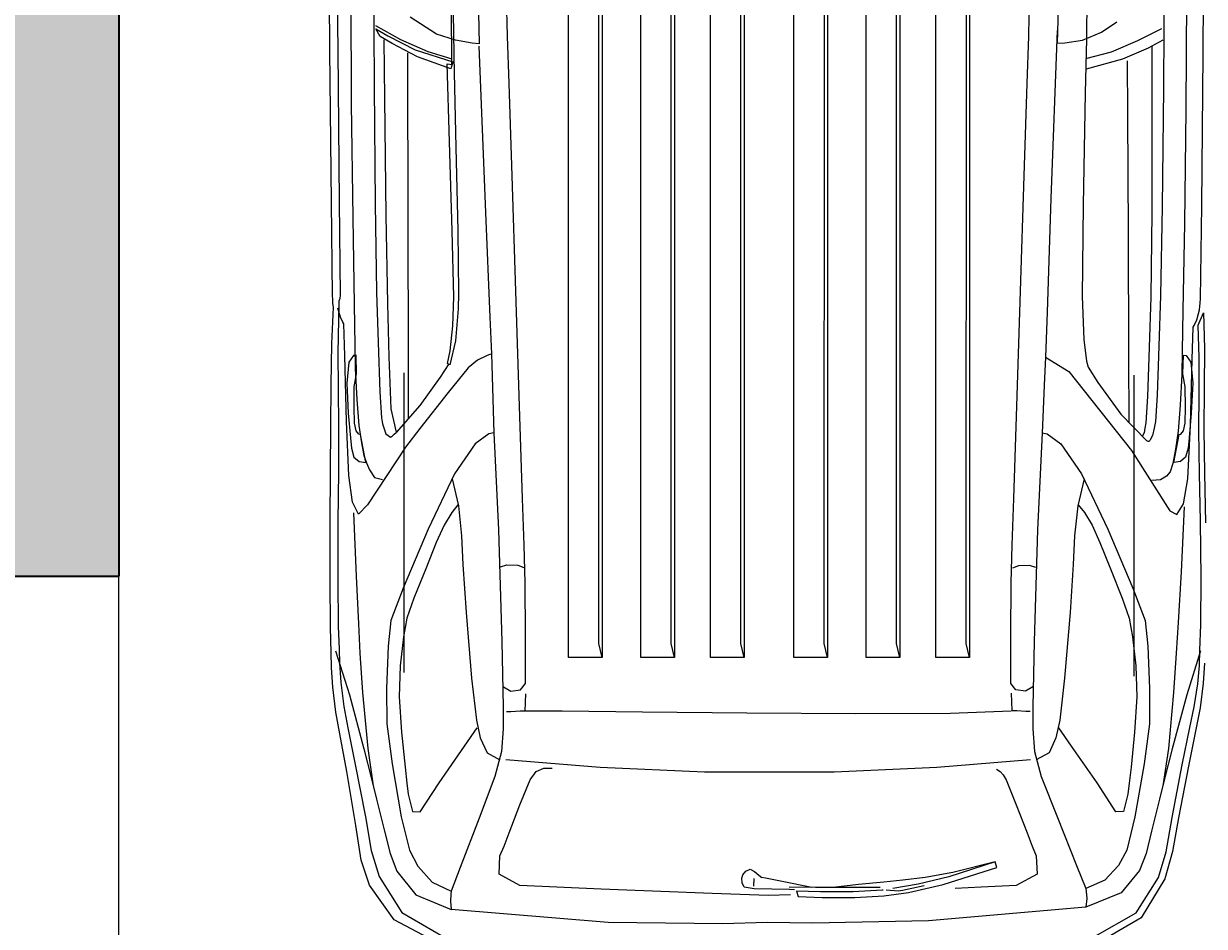
# Model space of a CAD drawing. Units: inches. Extents: x -16 to 587, y -783 to 64.
# Tile 3 of 14: x 111 to 195, y -697 to -633. Entities that reach past the tile are written whole.
import ezdxf

# ---------------------------------------------------------------- set-up
doc = ezdxf.new("R2010")
doc.units = ezdxf.units.IN
doc.header["$MEASUREMENT"] = 0
for name, color, linetype, lineweight in [('A-ANNO-DIMS', 2, 'Continuous', 18), ('A-SITE-VEHC', 8, 'Continuous', 13), ('A-WALL', 7, 'Continuous', 35), ('A-WALL-PATT', 23, 'Continuous', 13)]:
    doc.layers.add(name, color=color, linetype=linetype, lineweight=lineweight)
doc.styles.get("Standard").update_dxf_attribs({"font": 'arial.ttf'})
doc.dimstyles.get("Standard").update_dxf_attribs({"dimtxt": 0.18, "dimasz": 0.18, "dimexe": 0.18, "dimexo": 0.0625, "dimgap": 0.09, "dimtad": 0, "dimtih": 1, "dimtoh": 1, "dimdec": 0, "dimzin": 0, "dimdsep": 46, "dimlunit": 3, "dimtxsty": 'Standard', "dimcen": 0.09, "dimadec": 0, "dimazin": 0, "dimtfac": 1, "dimtdec": 0, "dimtofl": 0, "dimtmove": 0, "dimatfit": 3, "dimfxl": 1, "dimtolj": 1, "dimtzin": 0, "dimarcsym": 0})

# ---------------------------------------------------------------- blocks, each defined once
blk = doc.blocks.new('*D56')
at = {"layer": 'A-ANNO-DIMS', "color": 0, "lineweight": -2, "transparency": 16777216}
for p, q in [((118.083, -728.492), (118.083, 63.775)), ((228.083, -728.492), (228.083, 63.775)), ((118.263, 63.595), (172.753, 63.595)), ((227.903, 63.595), (173.412, 63.595))]:
    blk.add_line(p, q, dxfattribs=at)
at = {"layer": 'A-ANNO-DIMS', "color": 0, "transparency": 16777216}
for points in [[(118.263, 63.625), (118.263, 63.565), (118.083, 63.595)], [(227.903, 63.625), (227.903, 63.565), (228.083, 63.595)]]:
    blk.add_solid(points, dxfattribs=at)
at = {"layer": 'Defpoints', "color": 0, "transparency": 16777216}
for p in [(228.083, 63.595), (118.083, -728.555), (228.083, -728.555)]:
    blk.add_point(p, dxfattribs=at)
at = {"layer": 'A-ANNO-DIMS', "color": 0, "transparency": 16777216, "insert": (173.083, 63.595), "char_height": 0.18, "attachment_point": 5}
blk.add_mtext('\\A1;9\'-2"', dxfattribs=at)

msp = doc.modelspace()

# ---------------------------------------------------------------- hatches: boundary and pattern name
at = {"layer": 'A-WALL-PATT'}
h = msp.add_hatch(color=256, dxfattribs=at)
h.dxf.hatch_style = 1
h.paths.add_polyline_path([(137.083, -543.555), (137.083, -534.555), (118.083, -534.555), (118.083, -528.555), (109.083, -528.555), (109.083, -534.555), (109.083, -672.555), (118.083, -672.555), (118.083, -543.555)], flags=17)
h.paths.add_polyline_path([(27.083, -663.555), (27.083, -400.555), (73.083, -400.555), (73.083, -391.555), (27.083, -391.555), (27.083, 10.445), (48.751, 10.445), (171.083, 10.445), (171.083, -17.555), (180.083, -17.555), (180.083, 10.445), (228.083, 10.445), (228.083, -262.555), (206.414, -262.555), (118.083, -262.555), (118.083, -271.555), (228.083, -271.555), (228.083, -391.555), (154.083, -391.555), (154.083, -400.555), (228.083, -400.555), (228.083, -534.555), (209.083, -534.555), (209.083, -543.555), (237.083, -543.555), (237.083, 19.445), (18.083, 19.445), (18.083, -672.555), (73.083, -672.555), (73.083, -663.555)])
h.paths.add_polyline_path([(109.083, -486.555), (87.083, -486.555), (87.083, -495.555), (118.083, -495.555), (118.083, -400.555), (118.083, -391.555), (109.083, -391.555), (109.083, -400.555)], flags=17)

# ---------------------------------------------------------------- linework, layer by layer
at = {"layer": 'A-SITE-VEHC'}
for p, q in [((149.989, -678.315), (149.989, -615.867)), ((152.131, -677.322), (152.153, -616.064)), ((152.368, -615.867), (152.368, -678.315)), ((152.369, -615.867), (152.369, -678.315)), ((155.117, -678.315), (155.117, -615.867)), ((157.258, -677.322), (157.281, -616.064)), ((157.495, -615.867), (157.495, -678.315)), ((157.497, -615.867), (157.497, -678.315)), ((160.061, -678.315), (160.061, -615.867)), ((162.203, -677.322), (162.226, -616.064)), ((162.44, -615.867), (162.44, -678.315)), ((162.442, -615.867), (162.442, -678.315)), ((165.977, -678.315), (165.977, -615.867)), ((168.119, -677.322), (168.142, -616.064)), ((168.355, -615.867), (168.355, -678.315)), ((168.358, -615.867), (168.358, -678.315)), ((171.105, -678.315), (171.105, -615.867)), ((173.247, -677.322), (173.269, -616.064)), ((173.483, -615.867), (173.483, -678.315)), ((173.485, -615.867), (173.485, -678.315)), ((176.049, -678.315), (176.049, -615.867)), ((178.193, -677.322), (178.216, -616.064)), ((178.43, -615.867), (178.43, -678.315)), ((136.149, -628.168), (136.172, -633.662)), ((143.513, -627.927), (143.651, -634.79)), ((184.831, -628.18), (184.658, -634.742)), ((186.781, -628.18), (186.726, -634.447)), ((192.201, -628.493), (192.219, -633.733)), ((133.062, -635.266), (133.014, -629.627)), ((133.563, -629.627), (133.612, -635.26)), ((134.53, -630.409), (134.576, -639.048)), ((195.007, -635.526), (195.055, -629.894)), ((145.651, -634.256), (145.592, -631.197)), ((182.649, -634.256), (182.694, -631.197)), ((193.822, -630.822), (193.776, -639.461)), ((141.7, -636.249), (141.678, -632.257)), ((141.81, -632.032), (141.839, -634.647)), ((140.613, -634.097), (138.765, -632.909)), ((187.79, -633.974), (188.879, -633.219)), ((136.172, -633.662), (136.195, -637.823)), ((136.3, -633.494), (138.077, -634.49)), ((136.629, -634.28), (136.309, -633.731)), ((136.309, -633.731), (137.18, -634.234)), ((184.654, -633.854), (184.211, -645.765)), ((186.45, -634.523), (187.79, -633.974)), ((192.055, -633.715), (190.357, -634.583)), ((192.219, -633.733), (192.184, -637.941)), ((137.472, -634.762), (136.629, -634.28)), ((136.881, -634.509), (136.926, -638.662)), ((137.18, -634.234), (139.112, -635.22)), ((139.269, -635.713), (137.472, -634.762)), ((138.077, -634.49), (139.998, -635.336)), ((141.97, -634.541), (140.613, -634.097)), ((141.839, -634.647), (141.844, -634.913)), ((141.844, -634.913), (141.858, -635.662)), ((143.148, -634.743), (141.97, -634.541)), ((143.651, -634.79), (143.148, -634.743)), ((145.773, -637.594), (145.651, -634.256)), ((182.528, -637.594), (182.649, -634.256)), ((184.658, -634.742), (185.206, -634.718)), ((185.206, -634.718), (186.45, -634.523)), ((186.726, -634.447), (186.648, -638.301)), ((190.357, -634.583), (188.471, -635.385)), ((191.135, -635.064), (192.159, -634.504)), ((133.163, -646.019), (133.062, -635.266)), ((133.612, -635.26), (133.712, -646.003)), ((138.575, -635.425), (138.591, -647.803)), ((139.112, -635.22), (141.791, -636.078)), ((141.632, -636.568), (139.269, -635.713)), ((139.998, -635.336), (141.711, -635.86)), ((141.858, -635.662), (141.879, -636.817)), ((143.633, -634.947), (144.098, -646.751)), ((188.471, -635.385), (186.667, -635.865)), ((189.312, -635.852), (191.135, -635.064)), ((191.363, -634.99), (191.372, -638.895)), ((194.907, -646.267), (195.007, -635.526)), ((141.541, -641.747), (141.368, -636.203)), ((141.368, -636.203), (141.7, -636.249)), ((141.791, -636.078), (141.632, -636.568)), ((186.726, -636.575), (189.312, -635.852)), ((189.624, -635.997), (189.641, -639.778)), ((141.879, -636.817), (141.997, -642.132)), ((136.195, -637.823), (136.26, -646.146)), ((145.986, -644.154), (145.773, -637.594)), ((182.315, -644.154), (182.528, -637.594)), ((192.184, -637.941), (192.096, -646.352)), ((134.576, -639.048), (134.677, -647.128)), ((136.926, -638.662), (137.032, -646.97)), ((186.648, -638.301), (186.504, -646.213)), ((191.372, -638.895), (191.366, -646.746)), ((189.641, -639.778), (189.68, -648.216)), ((193.776, -639.461), (193.674, -647.541)), ((141.737, -648.057), (141.541, -641.747)), ((141.997, -642.132), (142.129, -648.027)), ((146.246, -652.323), (145.986, -644.154)), ((182.055, -652.323), (182.315, -644.154)), ((184.211, -645.765), (183.932, -653.817)), ((133.251, -652.643), (133.163, -646.019)), ((133.712, -646.003), (133.8, -652.621)), ((136.26, -646.146), (136.362, -652.395)), ((186.504, -646.213), (186.427, -652.707)), ((192.096, -646.352), (191.982, -652.648)), ((194.819, -652.885), (194.907, -646.267)), ((134.677, -647.128), (134.779, -653.29)), ((137.032, -646.97), (137.156, -653.211)), ((144.098, -646.751), (144.407, -654.185)), ((191.366, -646.746), (191.295, -652.74)), ((138.591, -647.803), (138.603, -656.65)), ((141.849, -652.731), (141.737, -648.057)), ((142.129, -648.027), (142.192, -652.466)), ((189.68, -648.216), (189.719, -656.953)), ((193.674, -647.541), (193.573, -653.703)), ((136.362, -652.395), (136.48, -655.983)), ((142.192, -652.466), (142.151, -653.59)), ((146.506, -660.487), (146.246, -652.323)), ((181.795, -660.487), (182.055, -652.323)), ((133.259, -652.922), (133.251, -652.643)), ((133.272, -653.202), (133.259, -652.922)), ((133.306, -653.479), (133.272, -653.202)), ((133.699, -653.28), (133.676, -654.356)), ((133.705, -653.053), (133.699, -653.28)), ((133.767, -652.85), (133.705, -653.053)), ((133.8, -652.621), (133.767, -652.85)), ((134.779, -653.29), (134.825, -656.178)), ((137.156, -653.211), (137.246, -656.981)), ((141.779, -654.797), (141.849, -652.731)), ((186.427, -652.707), (186.534, -655.77)), ((191.295, -652.74), (191.177, -656.327)), ((191.982, -652.648), (191.864, -656.236)), ((194.776, -653.424), (194.802, -653.167)), ((194.802, -653.167), (194.819, -652.885)), ((133.208, -656.064), (133.306, -653.479)), ((133.807, -654.176), (133.626, -653.534)), ((133.98, -654.532), (133.807, -654.176)), ((142.151, -653.59), (141.974, -655.847)), ((183.932, -653.817), (183.827, -657.007)), ((193.573, -653.703), (193.527, -656.591)), ((194.557, -654.376), (194.742, -653.659)), ((194.66, -654.745), (195.036, -653.862)), ((194.742, -653.659), (194.776, -653.424)), ((195.036, -653.862), (195.093, -656.392)), ((133.676, -654.356), (133.624, -656.711)), ((134.057, -654.641), (133.98, -654.532)), ((134.109, -656.918), (134.057, -654.641)), ((141.592, -656.558), (141.779, -654.797)), ((144.407, -654.185), (144.518, -656.769)), ((194.235, -657.171), (194.287, -654.894)), ((194.287, -654.894), (194.371, -654.773)), ((194.371, -654.773), (194.557, -654.376)), ((194.724, -657.068), (194.66, -654.745)), ((141.974, -655.847), (141.574, -657.56)), ((186.534, -655.77), (186.733, -657.308)), ((133.148, -658.988), (133.208, -656.064)), ((134.825, -656.178), (134.862, -657.82)), ((136.48, -655.983), (136.598, -659.466)), ((138.603, -656.65), (138.608, -661.379)), ((141.391, -657.469), (141.592, -656.558)), ((191.177, -656.327), (191.059, -659.81)), ((191.864, -656.236), (191.746, -659.719)), ((193.527, -656.591), (193.489, -658.233)), ((195.093, -656.392), (195.072, -659.213)), ((133.624, -656.711), (133.652, -659.212)), ((134.241, -661.585), (134.109, -656.918)), ((134.405, -657.373), (134.258, -658.856)), ((134.739, -656.903), (134.405, -657.373)), ((134.924, -656.874), (134.739, -656.903)), ((134.957, -658.2), (134.924, -656.874)), ((137.246, -656.981), (137.389, -660.687)), ((141.504, -657.478), (140.893, -658.423)), ((141.574, -657.56), (141.391, -657.469)), ((143.54, -657.231), (142.863, -657.774)), ((144.169, -656.915), (143.54, -657.231)), ((144.446, -656.813), (144.169, -656.915)), ((144.518, -656.769), (144.7, -662.379)), ((183.827, -657.007), (183.737, -659.007)), ((183.827, -657.007), (185.481, -658.027)), ((186.733, -657.308), (186.84, -657.731)), ((189.719, -656.953), (189.736, -661.632)), ((193.573, -658.2), (193.607, -656.874)), ((193.607, -656.874), (193.792, -656.903)), ((193.792, -656.903), (194.125, -657.373)), ((194.103, -661.837), (194.235, -657.171)), ((194.125, -657.373), (194.273, -658.856)), ((194.72, -659.512), (194.724, -657.068)), ((134.789, -659.128), (134.957, -658.2)), ((134.862, -657.82), (134.965, -660.013)), ((138.299, -658.133), (138.299, -679.377)), ((142.863, -657.774), (141.451, -659.518)), ((185.481, -658.027), (189.913, -663.641)), ((186.84, -657.731), (187.545, -658.817)), ((190.084, -658.285), (190.084, -679.645)), ((193.489, -658.233), (193.387, -660.426)), ((193.741, -659.128), (193.573, -658.2)), ((133.129, -661.962), (133.148, -658.988)), ((134.258, -658.856), (134.367, -660.989)), ((134.783, -660.566), (134.789, -659.128)), ((140.893, -658.423), (139.45, -660.453)), ((183.737, -659.007), (183.634, -661.29)), ((187.545, -658.817), (189.169, -661.058)), ((193.748, -660.566), (193.741, -659.128)), ((194.273, -658.856), (194.164, -660.989)), ((133.652, -659.212), (133.678, -661.962)), ((134.965, -660.013), (135.121, -661.852)), ((136.598, -659.466), (136.716, -661.32)), ((141.451, -659.518), (139.448, -662.077)), ((191.059, -659.81), (190.941, -661.664)), ((191.746, -659.719), (191.628, -661.573)), ((194.706, -662.231), (194.72, -659.512)), ((195.072, -659.213), (195.049, -662.139)), ((134.809, -661.704), (134.783, -660.566)), ((137.389, -660.687), (137.751, -662.323)), ((139.45, -660.453), (137.754, -662.366)), ((146.72, -667.033), (146.506, -660.487)), ((181.581, -667.033), (181.795, -660.487)), ((193.387, -660.426), (193.231, -662.265)), ((193.722, -661.704), (193.748, -660.566)), ((134.412, -665.398), (134.241, -661.585)), ((134.367, -660.989), (134.512, -662.738)), ((134.916, -662.248), (134.809, -661.704)), ((136.716, -661.32), (136.794, -661.737)), ((183.634, -661.29), (183.584, -662.379)), ((189.169, -661.058), (190.978, -662.932)), ((190.941, -661.664), (190.88, -662.049)), ((191.628, -661.573), (191.533, -662.053)), ((193.615, -662.248), (193.722, -661.704)), ((194.164, -660.989), (194.019, -662.738)), ((133.113, -665.101), (133.129, -661.962)), ((133.678, -661.962), (133.663, -665.101)), ((135.115, -662.466), (134.916, -662.248)), ((135.221, -662.505), (135.115, -662.466)), ((135.121, -661.852), (135.298, -663.08)), ((135.61, -664.497), (135.221, -662.505)), ((136.794, -661.737), (137.017, -662.456)), ((137.017, -662.456), (137.367, -662.679)), ((137.493, -662.585), (137.623, -662.48)), ((137.623, -662.48), (137.754, -662.366)), ((139.448, -662.077), (138.431, -663.388)), ((144.346, -662.447), (143.37, -663.163)), ((144.7, -662.379), (144.346, -662.447)), ((144.7, -662.379), (145.028, -669.269)), ((183.584, -662.379), (183.256, -669.269)), ((183.584, -662.379), (183.939, -662.447)), ((183.939, -662.447), (184.915, -663.163)), ((190.821, -662.384), (190.677, -662.643)), ((190.88, -662.049), (190.821, -662.384)), ((191.533, -662.053), (191.41, -662.566)), ((192.92, -664.497), (193.309, -662.505)), ((193.231, -662.265), (193.046, -663.548)), ((193.309, -662.505), (193.416, -662.466)), ((193.416, -662.466), (193.615, -662.248)), ((193.932, -665.651), (194.103, -661.837)), ((194.747, -665.254), (194.706, -662.231)), ((195.049, -662.139), (195.092, -665.231)), ((134.512, -662.738), (134.584, -663.462)), ((135.298, -663.08), (135.475, -663.992)), ((138.431, -663.388), (135.737, -667.496)), ((137.367, -662.679), (137.493, -662.585)), ((143.37, -663.163), (141.906, -665.292)), ((184.915, -663.163), (186.379, -665.292)), ((190.978, -662.932), (191.072, -662.976)), ((191.072, -662.976), (191.157, -662.97)), ((191.157, -662.97), (191.231, -662.921)), ((191.41, -662.566), (191.231, -662.921)), ((194.019, -662.738), (193.947, -663.462)), ((134.584, -663.462), (134.769, -664.1)), ((134.769, -664.1), (135.126, -664.407)), ((135.475, -663.992), (135.653, -664.511)), ((189.913, -663.641), (192.645, -667.908)), ((193.046, -663.548), (192.854, -664.564)), ((193.761, -664.1), (193.404, -664.407)), ((193.947, -663.462), (193.761, -664.1)), ((135.126, -664.407), (135.61, -664.497)), ((135.653, -664.511), (135.874, -664.998)), ((135.874, -664.998), (136.229, -665.55)), ((192.854, -664.564), (192.668, -665.138)), ((193.404, -664.407), (192.92, -664.497)), ((133.085, -668.714), (133.113, -665.101)), ((133.663, -665.101), (133.634, -668.714)), ((134.666, -667.307), (134.412, -665.398)), ((136.229, -665.55), (136.79, -665.687)), ((141.906, -665.292), (140.034, -669.218)), ((141.727, -665.649), (142.179, -667.552)), ((186.557, -665.649), (186.106, -667.552)), ((186.379, -665.292), (188.251, -669.218)), ((191.988, -665.712), (191.363, -665.756)), ((192.414, -665.455), (191.988, -665.712)), ((192.668, -665.138), (192.414, -665.455)), ((193.617, -667.426), (193.932, -665.651)), ((194.824, -668.655), (194.747, -665.254)), ((195.092, -665.231), (195.172, -668.76)), ((135.097, -668.146), (134.666, -667.307)), ((135.737, -667.496), (135.097, -668.146)), ((142.143, -667.492), (141.703, -668.027)), ((142.179, -667.552), (142.406, -669.692)), ((146.841, -670.346), (146.72, -667.033)), ((181.46, -670.346), (181.581, -667.033)), ((186.106, -667.552), (185.879, -669.692)), ((186.141, -667.492), (186.581, -668.027)), ((193.133, -668.165), (193.617, -667.426)), ((134.729, -668.045), (134.914, -672.546)), ((141.703, -668.027), (141.157, -668.919)), ((186.581, -668.027), (187.128, -668.919)), ((192.645, -667.908), (193.133, -668.165)), ((193.653, -667.633), (193.443, -672.241)), ((133.069, -672.843), (133.085, -668.714)), ((133.634, -668.714), (133.619, -672.843)), ((140.034, -669.218), (138.268, -673.396)), ((141.157, -668.919), (140.598, -670.168)), ((187.128, -668.919), (187.687, -670.168)), ((188.251, -669.218), (190.017, -673.396)), ((194.866, -672.669), (194.824, -668.655)), ((142.406, -669.692), (142.5, -671.714)), ((145.028, -669.269), (145.264, -677.19)), ((183.256, -669.269), (183.021, -677.19)), ((185.879, -669.692), (185.784, -671.714)), ((140.598, -670.168), (139.86, -672.017)), ((146.907, -673.014), (146.841, -670.346)), ((181.394, -673.014), (181.46, -670.346)), ((187.687, -670.168), (188.425, -672.017)), ((142.5, -671.714), (142.72, -675.136)), ((145.168, -671.891), (145.601, -671.753)), ((145.601, -671.753), (146.402, -671.759)), ((146.402, -671.759), (146.828, -671.925)), ((185.784, -671.714), (185.564, -675.136)), ((134.914, -672.546), (135.082, -675.933)), ((139.86, -672.017), (139.017, -674.105)), ((181.898, -671.805), (181.473, -671.971)), ((182.7, -671.798), (181.898, -671.805)), ((183.133, -671.937), (182.7, -671.798)), ((188.425, -672.017), (189.268, -674.105)), ((193.443, -672.241), (193.228, -675.826)), ((133.096, -676.179), (133.069, -672.843)), ((133.619, -672.843), (133.65, -676.1)), ((138.268, -673.396), (137.387, -675.697)), ((146.938, -676.737), (146.907, -673.014)), ((181.363, -676.737), (181.394, -673.014)), ((190.017, -673.396), (190.897, -675.697)), ((194.836, -676.009), (194.866, -672.669)), ((139.017, -674.105), (138.517, -675.519)), ((189.268, -674.105), (189.768, -675.519)), ((135.082, -675.933), (135.187, -678.016)), ((137.387, -675.697), (137.204, -677.514)), ((138.517, -675.519), (138.286, -676.849)), ((142.72, -675.136), (143.112, -679.786)), ((185.564, -675.136), (185.172, -679.786)), ((189.768, -675.519), (189.999, -676.849)), ((190.897, -675.697), (191.08, -677.514)), ((193.228, -675.826), (193.098, -678.016)), ((133.146, -677.957), (133.096, -676.179)), ((133.65, -676.1), (133.707, -677.732)), ((146.939, -680.172), (146.938, -676.737)), ((181.362, -680.172), (181.363, -676.737)), ((194.781, -677.793), (194.836, -676.009)), ((137.204, -677.514), (137.074, -680.519)), ((138.286, -676.849), (138.054, -678.905)), ((145.264, -677.19), (145.354, -681.821)), ((152.368, -678.315), (152.131, -677.322)), ((157.495, -678.315), (157.258, -677.322)), ((162.44, -678.315), (162.203, -677.322)), ((168.355, -678.315), (168.119, -677.322)), ((173.483, -678.315), (173.247, -677.322)), ((178.43, -678.315), (178.193, -677.322)), ((183.021, -677.19), (182.93, -681.821)), ((189.999, -676.849), (190.23, -678.905)), ((191.08, -677.514), (191.21, -680.519)), ((133.173, -679.033), (133.146, -677.957)), ((133.463, -677.837), (134.443, -680.962)), ((133.707, -677.732), (133.738, -678.729)), ((135.187, -678.016), (135.381, -680.808)), ((152.369, -678.315), (149.989, -678.315)), ((157.497, -678.315), (155.117, -678.315)), ((162.442, -678.315), (160.061, -678.315)), ((168.358, -678.315), (165.977, -678.315)), ((173.485, -678.315), (171.105, -678.315)), ((178.43, -678.315), (176.049, -678.315)), ((193.098, -678.016), (192.904, -680.808)), ((194.822, -677.837), (193.842, -680.962)), ((194.751, -678.873), (194.781, -677.793)), ((133.262, -680.431), (133.173, -679.033)), ((133.738, -678.729), (133.825, -680.08)), ((138.054, -678.905), (137.982, -681.107)), ((190.23, -678.905), (190.303, -681.107)), ((194.638, -680.183), (194.751, -678.873)), ((195.096, -678.729), (195.007, -680.127)), ((133.825, -680.08), (134.042, -681.789)), ((143.112, -679.786), (143.452, -682.772)), ((185.172, -679.786), (184.833, -682.772)), ((195.007, -680.127), (194.784, -681.879)), ((133.485, -682.183), (133.262, -680.431)), ((134.443, -680.962), (135.476, -684.8)), ((135.381, -680.808), (135.746, -684.776)), ((137.074, -680.519), (137.09, -683.01)), ((145.378, -680.4), (145.888, -680.709)), ((145.888, -680.709), (146.587, -680.61)), ((146.587, -680.61), (146.939, -680.172)), ((146.939, -680.899), (146.9, -682.118)), ((181.714, -680.61), (181.362, -680.172)), ((181.397, -680.848), (181.436, -682.068)), ((182.413, -680.709), (181.714, -680.61)), ((182.923, -680.4), (182.413, -680.709)), ((191.21, -680.519), (191.195, -683.01)), ((192.904, -680.808), (192.538, -684.776)), ((193.842, -680.962), (192.809, -684.8)), ((194.373, -681.818), (194.638, -680.183)), ((134.042, -681.789), (134.325, -683.303)), ((137.982, -681.107), (138.147, -683.62)), ((145.354, -681.821), (145.359, -683.365)), ((182.93, -681.821), (182.926, -683.365)), ((190.303, -681.107), (190.138, -683.62)), ((194.065, -683.291), (194.373, -681.818)), ((133.775, -683.735), (133.485, -682.183)), ((145.905, -682.162), (145.592, -682.178)), ((146.548, -682.134), (145.905, -682.162)), ((146.9, -682.118), (146.548, -682.134)), ((149.539, -682.131), (146.9, -682.118)), ((155.239, -682.197), (149.539, -682.131)), ((162.637, -682.274), (155.239, -682.197)), ((170.37, -682.316), (162.637, -682.274)), ((177.073, -682.279), (170.37, -682.316)), ((181.384, -682.118), (177.073, -682.279)), ((181.436, -682.068), (181.789, -682.083)), ((181.789, -682.083), (182.432, -682.112)), ((182.432, -682.112), (182.744, -682.127)), ((194.784, -681.879), (194.494, -683.43)), ((134.325, -683.303), (134.864, -685.906)), ((137.09, -683.01), (137.466, -685.866)), ((142.608, -684.598), (143.511, -683.307)), ((143.452, -682.772), (143.725, -684.012)), ((145.359, -683.365), (145.231, -684.974)), ((182.926, -683.365), (183.054, -684.974)), ((184.833, -682.772), (184.56, -684.012)), ((185.676, -684.598), (184.774, -683.307)), ((191.195, -683.01), (190.818, -685.866)), ((193.525, -685.921), (194.065, -683.291)), ((194.494, -683.43), (193.959, -686.016)), ((134.273, -686.4), (133.775, -683.735)), ((138.147, -683.62), (138.391, -686.106)), ((143.725, -684.012), (144.209, -685.08)), ((184.56, -684.012), (184.076, -685.08)), ((190.138, -683.62), (189.893, -686.106)), ((135.476, -684.8), (136.02, -686.934)), ((135.746, -684.776), (136.138, -687.41)), ((140.807, -687.209), (142.608, -684.598)), ((144.209, -685.08), (145.116, -685.567)), ((145.231, -684.974), (144.76, -686.756)), ((183.054, -684.974), (183.525, -686.756)), ((184.076, -685.08), (183.168, -685.567)), ((187.478, -687.209), (185.676, -684.598)), ((192.538, -684.776), (192.146, -687.41)), ((192.809, -684.8), (192.265, -686.934)), ((134.864, -685.906), (135.575, -689.609)), ((137.466, -685.866), (138.12, -689.608)), ((152.225, -686.128), (145.532, -685.567)), ((182.752, -685.567), (176.122, -686.128)), ((190.818, -685.866), (190.164, -689.608)), ((192.813, -689.674), (193.525, -685.921)), ((134.909, -690.228), (134.273, -686.4)), ((138.391, -686.106), (138.517, -687.231)), ((144.76, -686.756), (143.641, -689.711)), ((147.257, -686.994), (147.685, -686.399)), ((147.685, -686.399), (148.228, -686.165)), ((148.228, -686.165), (148.83, -686.159)), ((159.63, -686.452), (152.225, -686.128)), ((164.261, -686.458), (159.63, -686.452)), ((168.831, -686.452), (164.261, -686.458)), ((176.122, -686.128), (168.831, -686.452)), ((180.337, -686.245), (180.599, -686.398)), ((180.599, -686.398), (180.831, -686.642)), ((180.831, -686.642), (181.028, -686.994)), ((183.525, -686.756), (184.663, -689.664)), ((189.893, -686.106), (189.768, -687.231)), ((193.959, -686.016), (193.252, -689.694)), ((136.02, -686.934), (136.372, -688.359)), ((138.517, -687.231), (138.618, -688.007)), ((139.468, -689.253), (140.807, -687.209)), ((146.541, -688.766), (147.257, -686.994)), ((181.028, -686.994), (181.744, -688.766)), ((188.817, -689.253), (187.478, -687.209)), ((189.768, -687.231), (189.667, -688.007)), ((192.265, -686.934), (191.913, -688.359)), ((136.372, -688.359), (136.936, -690.642)), ((138.618, -688.007), (138.931, -689.231)), ((189.667, -688.007), (189.354, -689.231)), ((191.913, -688.359), (191.349, -690.642)), ((138.931, -689.231), (139.468, -689.253)), ((145.773, -690.751), (146.541, -688.766)), ((181.744, -688.766), (182.512, -690.751)), ((189.354, -689.231), (188.817, -689.253)), ((135.575, -689.609), (135.995, -692.013)), ((138.12, -689.608), (138.695, -691.988)), ((143.641, -689.711), (142.311, -693.207)), ((184.663, -689.664), (186.031, -693.071)), ((190.164, -689.608), (189.59, -691.988)), ((192.393, -692.104), (192.813, -689.674)), ((193.252, -689.694), (192.835, -692.082)), ((135.289, -692.696), (134.909, -690.228)), ((136.936, -690.642), (137.328, -692.226)), ((145.414, -691.691), (145.773, -690.751)), ((182.512, -690.751), (182.871, -691.691)), ((191.349, -690.642), (190.957, -692.226)), ((145.112, -692.376), (145.414, -691.691)), ((182.871, -691.691), (183.173, -692.376)), ((135.879, -694.476), (135.289, -692.696)), ((135.995, -692.013), (136.555, -693.85)), ((137.328, -692.226), (137.815, -693.481)), ((138.695, -691.988), (139.307, -693.111)), ((145.061, -693.681), (145.112, -692.376)), ((183.173, -692.376), (183.223, -693.681)), ((189.59, -691.988), (188.997, -693.064)), ((190.957, -692.226), (190.49, -693.434)), ((191.845, -693.911), (192.393, -692.104)), ((192.835, -692.082), (192.287, -694.021)), ((137.815, -693.481), (139.148, -695.144)), ((139.307, -693.111), (140.303, -694.246)), ((142.311, -693.207), (141.668, -694.894)), ((162.353, -693.728), (162.566, -693.46)), ((162.566, -693.46), (162.864, -693.341)), ((162.864, -693.341), (163.191, -693.491)), ((163.191, -693.491), (163.487, -693.758)), ((176.562, -694.423), (180.376, -693.208)), ((180.256, -692.813), (176.975, -693.871)), ((180.256, -692.813), (177.239, -693.57)), ((180.376, -693.208), (180.256, -692.813)), ((186.031, -693.071), (186.694, -694.711)), ((188.997, -693.064), (188.039, -694.111)), ((190.49, -693.434), (189.194, -695.008)), ((136.555, -693.85), (138.168, -696.408)), ((140.303, -694.246), (141.668, -694.894)), ((146.543, -694.485), (145.061, -693.681)), ((162.291, -693.959), (162.353, -693.728)), ((162.302, -694.305), (162.291, -693.959)), ((162.456, -694.61), (162.302, -694.305)), ((163.125, -694.528), (163.163, -693.99)), ((163.487, -693.758), (163.702, -693.922)), ((163.966, -693.968), (163.702, -693.922)), ((165.02, -694.17), (163.966, -693.968)), ((167.257, -694.625), (165.02, -694.17)), ((172.361, -694.247), (170.563, -694.411)), ((173.699, -694.118), (172.361, -694.247)), ((175.28, -693.925), (173.699, -694.118)), ((176.975, -693.871), (174.794, -694.394)), ((177.239, -693.57), (175.28, -693.925)), ((183.223, -693.681), (181.741, -694.485)), ((188.039, -694.111), (186.694, -694.711)), ((190.25, -696.415), (191.845, -693.911)), ((192.287, -694.021), (190.62, -696.776)), ((137.623, -696.935), (135.879, -694.476)), ((139.148, -695.144), (141.668, -696.202)), ((141.641, -695.101), (141.615, -695.599)), ((141.668, -694.894), (141.641, -695.101)), ((152.295, -694.749), (146.543, -694.485)), ((160.174, -695.053), (152.295, -694.749)), ((164.142, -695.199), (160.174, -695.053)), ((163.168, -694.719), (162.456, -694.61)), ((165.664, -694.78), (163.168, -694.719)), ((165.725, -695.141), (164.142, -695.199)), ((167.503, -694.621), (165.64, -694.612)), ((166.017, -694.784), (165.664, -694.78)), ((167.852, -694.934), (166.163, -694.882)), ((166.163, -694.882), (166.283, -695.277)), ((170.521, -694.628), (167.503, -694.621)), ((170.172, -694.935), (167.852, -694.934)), ((170.563, -694.411), (168.756, -694.621)), ((172.226, -694.82), (170.172, -694.935)), ((170.293, -695.33), (172.346, -695.215)), ((172.102, -694.631), (170.521, -694.628)), ((172.249, -694.817), (172.226, -694.82)), ((172.272, -694.815), (172.249, -694.817)), ((172.296, -694.812), (172.272, -694.815)), ((172.346, -695.215), (174.102, -694.978)), ((173.399, -694.896), (172.53, -694.83)), ((174.794, -694.394), (172.992, -694.707)), ((173.669, -694.845), (173.399, -694.896)), ((174.344, -694.707), (173.669, -694.845)), ((174.102, -694.978), (176.562, -694.423)), ((175.217, -694.503), (174.344, -694.707)), ((179.257, -694.611), (177.418, -694.691)), ((180.738, -694.541), (179.257, -694.611)), ((181.741, -694.485), (180.738, -694.541)), ((186.694, -694.711), (186.72, -694.918)), ((189.194, -695.008), (186.694, -696.019)), ((186.72, -694.918), (186.746, -695.416)), ((141.615, -695.599), (141.668, -696.202)), ((166.283, -695.277), (167.972, -695.329)), ((167.972, -695.329), (170.293, -695.33)), ((186.694, -696.019), (175.52, -696.987)), ((186.746, -695.416), (186.694, -696.019)), ((138.168, -696.408), (141.093, -698.102)), ((152.791, -697.122), (141.668, -696.202)), ((187.336, -698.08), (190.25, -696.415)), ((190.62, -696.776), (187.443, -698.619)), ((140.841, -698.619), (137.623, -696.935)), ((160.927, -697.212), (152.791, -697.122)), ((164.083, -697.101), (160.927, -697.212)), ((167.289, -697.164), (164.083, -697.101)), ((175.52, -696.987), (167.289, -697.164))]:
    msp.add_line(p, q, dxfattribs=at)
at = {"layer": 'A-WALL'}
for p in [(118.083, -543.555), (109.083, -672.555)]:
    msp.add_line(p, (118.083, -672.555), dxfattribs=at)

# ---------------------------------------------------------------- dimensions: what is measured, and where the dimension line sits
at = {"layer": 'A-ANNO-DIMS'}
dim = msp.add_linear_dim(base=(228.083, 63.595), p1=(118.083, -728.555), p2=(228.083, -728.555), dimstyle='Standard', override={"dimdec": 1, "dimlfac": 1, "dimrnd": 0, "dimzin": 1, "dimdsep": 46, "dimlunit": 4, "dimfrac": 2}, dxfattribs=at)
dim.commit()
dim.dimension.update_dxf_attribs({"geometry": '*D56', "text_midpoint": (173.083, 63.595)})

doc.saveas('drawing.dxf')
